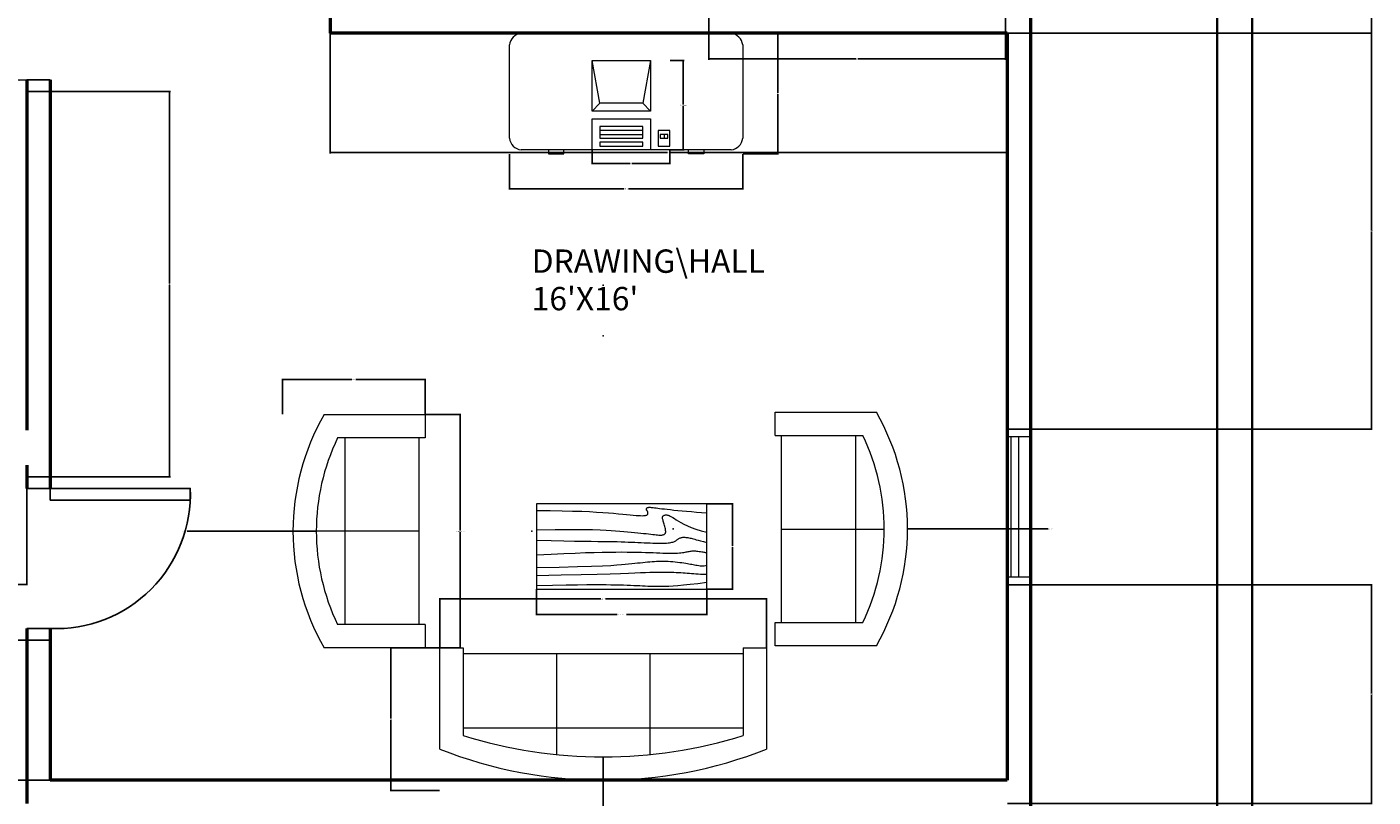
# Model space of a CAD drawing. Units: inches. Extents: x 156 to 720, y 11 to 679.
# Tile 3 of 5: x 374 to 720, y 161 to 359. Entities that reach past the tile are written whole.
import ezdxf

# ---------------------------------------------------------------- set-up
doc = ezdxf.new("R2010")
doc.units = ezdxf.units.IN
for name, color, linetype, lineweight in [('A-ANNO-DIMS', 2, 'Continuous', 18), ('A-AREA-IDEN', 7, 'Continuous', 25), ('A-DOOR', 3, 'Continuous', 25), ('A-EQPM', 9, 'Continuous', 13), ('A-FURN', 8, 'Continuous', 18), ('A-GLAZ', 4, 'Continuous', 18), ('A-WALL', 7, 'Continuous', 50), ('C-PROP', 7, 'Continuous', 35)]:
    doc.layers.add(name, color=color, linetype=linetype, lineweight=lineweight)
doc.styles.get("Standard").update_dxf_attribs({"font": 'arial.ttf'})
doc.dimstyles.get("Standard").update_dxf_attribs({"dimtxt": 0.18, "dimasz": 0.18, "dimexe": 0.18, "dimexo": 0.0625, "dimgap": 0.09, "dimtad": 0, "dimtih": 1, "dimtoh": 1, "dimdec": 4, "dimzin": 0, "dimdsep": 46, "dimtxsty": 'Standard', "dimcen": 0.09, "dimadec": 0, "dimazin": 0, "dimtfac": 1, "dimtdec": 4, "dimtofl": 0, "dimtmove": 0, "dimatfit": 3, "dimfxl": 1, "dimtolj": 1, "dimtzin": 0, "dimarcsym": 0})

# ---------------------------------------------------------------- blocks, each defined once
blk = doc.blocks.new('Sofa - Roundback Loveseat 5 ft.')
for p, q in [((0, -32.44198), (0, -5.99998)), ((-24, -33.99998), (-24, -11.46958)), ((-23.9998, -13.38178), (23.99986, -13.38178)), ((24.00004, -33.99998), (24.00004, -11.46958)), ((-24, -32.44198), (24.00004, -32.44198))]:
    blk.add_line(p, q)
for points in [[(-24, -33.99998), (-30, -33.99998), (-30, -7.99998)], [(30.00004, -7.99998), (30.00004, -33.99998), (24.00004, -33.99998)]]:
    blk.add_lwpolyline(points)
for centre, radius, start, end in [((0, -60.24998), 60.24998, 60.13715, 119.8628), ((0, -61.38438), 55.38444, 64.32083, 115.6792)]:
    blk.add_arc(centre, radius, start, end)
blk = doc.blocks.new('Table - Rectangular Woodgrain 60 x 30 in.')
for p, q in [((0, 0), (0, -30)), ((60, 0), (0, 0)), ((60, -30), (60, 0)), ((0, -30), (60, -30))]:
    blk.add_line(p, q)
for points in [[(0, -2.4), (4.8155, -2.418), (9.0302, -2.4688), (12.709, -2.5477), (15.9167, -2.65), (18.7181, -2.7711), (21.1781, -2.9063), (23.3616, -3.0508), (25.3333, -3.2), (27.1477, -3.3495), (28.8172, -3.4958), (30.3437, -3.636), (31.7291, -3.7667), (32.9756, -3.8849), (34.0849, -3.9875), (35.059, -4.0714), (35.9, -4.1334), (36.6114, -4.1711), (37.2041, -4.1854), (37.6906, -4.1779), (38.0833, -4.15), (38.3948, -4.1034), (38.6375, -4.0396), (38.8239, -3.9602), (38.9666, -3.8667), (39.0764, -3.7608), (39.1573, -3.6448), (39.2116, -3.521), (39.2416, -3.3917), (39.2498, -3.2593), (39.2385, -3.1261), (39.21, -2.9944), (39.1666, -2.8667), (39.111, -2.7447), (39.0468, -2.6281), (38.978, -2.5163), (38.9083, -2.4083), (38.8418, -2.3035), (38.7823, -2.201), (38.7337, -2.1001), (38.7, -2), (38.6844, -1.9003), (38.6875, -1.8021), (38.7094, -1.707), (38.75, -1.6167), (38.8094, -1.5326), (38.8875, -1.4563), (38.9844, -1.3893), (39.1, -1.3333), (39.2351, -1.2896), (39.3937, -1.2583), (39.5804, -1.2396), (39.8, -1.2333), (40.057, -1.2396), (40.3562, -1.2583), (40.7023, -1.2896), (41.1, -1.3333), (41.5547, -1.3895), (42.0755, -1.4573), (42.6721, -1.5361), (43.3542, -1.625), (44.1316, -1.7233), (45.014, -1.8302), (46.0114, -1.9449), (47.1333, -2.0667), (48.3862, -2.1947), (49.7625, -2.3281), (51.2513, -2.4663), (52.8416, -2.6083), (54.5226, -2.7535), (56.2833, -2.9011), (58.1127, -3.0501), (60, -3.2)], [(0, -9.2), (6.5759, -9.0858), (11.9385, -9.0365), (16.2527, -9.0418), (19.6833, -9.0917), (22.3952, -9.1759), (24.5531, -9.2844), (26.322, -9.4069), (27.8666, -9.5333), (29.3241, -9.6553), (30.7203, -9.7719), (32.0532, -9.8837), (33.3208, -9.9917), (34.5213, -10.0965), (35.6526, -10.199), (36.7128, -10.2999), (37.7, -10.4), (38.6129, -10.4996), (39.4531, -10.5969), (40.223, -10.6895), (40.925, -10.775), (41.5613, -10.8512), (42.1344, -10.9156), (42.6465, -10.966), (43.1, -11), (43.4976, -11.0158), (43.8437, -11.0136), (44.143, -10.9942), (44.4, -10.9583), (44.6195, -10.9069), (44.8062, -10.8406), (44.9648, -10.7603), (45.1, -10.6667), (45.2155, -10.5598), (45.3114, -10.4365), (45.3871, -10.2929), (45.4416, -10.125), (45.4743, -9.929), (45.4844, -9.7011), (45.4709, -9.4371), (45.4333, -9.1333), (45.3716, -8.7883), (45.2896, -8.4104), (45.1919, -8.0107), (45.0833, -7.6), (44.9685, -7.1893), (44.8521, -6.7896), (44.7388, -6.4117), (44.6333, -6.0667), (44.54, -5.7628), (44.4614, -5.4979), (44.4001, -5.2675), (44.3583, -5.0667), (44.3384, -4.8909), (44.3427, -4.7354), (44.3736, -4.5956), (44.4333, -4.4667), (44.5236, -4.3453), (44.6427, -4.2333), (44.7884, -4.1339), (44.9583, -4.05), (45.1501, -3.9849), (45.3614, -3.9417), (45.59, -3.9234), (45.8333, -3.9333), (46.0915, -3.9749), (46.3734, -4.0531), (46.6906, -4.1736), (47.0542, -4.3417), (47.4756, -4.5629), (47.9661, -4.8427), (48.5372, -5.1866), (49.2, -5.6), (49.9676, -6.0844), (50.8594, -6.625), (51.8965, -7.2031), (53.1, -7.8), (54.491, -8.3969), (56.0906, -8.975), (57.9199, -9.5156), (60, -10)], [(0, -12.8), (5.1847, -12.9322), (9.6213, -13.0323), (13.3963, -13.1059), (16.5958, -13.1583), (19.3063, -13.1952), (21.614, -13.2219), (23.6054, -13.2439), (25.3666, -13.2667), (26.9728, -13.2947), (28.4531, -13.3281), (29.8256, -13.3663), (31.1083, -13.4083), (32.3191, -13.4535), (33.476, -13.501), (34.597, -13.5501), (35.7, -13.6), (36.7984, -13.6497), (37.8875, -13.6979), (38.9578, -13.743), (40, -13.7833), (41.0047, -13.8174), (41.9625, -13.8438), (42.864, -13.8607), (43.7, -13.8667), (44.4631, -13.8604), (45.1552, -13.8417), (45.7801, -13.8104), (46.3416, -13.7667), (46.8439, -13.7104), (47.2906, -13.6417), (47.6858, -13.5604), (48.0333, -13.4667), (48.3375, -13.3608), (48.6042, -13.2448), (48.8396, -13.121), (49.05, -12.9917), (49.2417, -12.8593), (49.4208, -12.7261), (49.5937, -12.5944), (49.7667, -12.4667), (49.9452, -12.3451), (50.1323, -12.2313), (50.3303, -12.1268), (50.5416, -12.0333), (50.7686, -11.9524), (51.0135, -11.8854), (51.2788, -11.8341), (51.5666, -11.8), (51.8785, -11.7843), (52.2116, -11.7865), (52.562, -11.8059), (52.926, -11.8417), (53.2998, -11.8931), (53.6795, -11.9594), (54.0614, -12.0397), (54.4416, -12.1333), (54.8223, -12.2401), (55.2293, -12.3625), (55.6942, -12.5037), (56.2489, -12.6667), (56.9251, -12.8547), (57.7545, -13.0708), (58.7689, -13.3182), (60, -13.6)], [(0, -18), (5.124, -17.7273), (9.6609, -17.5057), (13.6705, -17.3303), (17.2125, -17.1958), (20.3467, -17.0973), (23.1328, -17.0297), (25.6307, -16.9878), (27.9, -16.9667), (29.9928, -16.9617), (31.9302, -16.9703), (33.7254, -16.9907), (35.3917, -17.0208), (36.9423, -17.0588), (38.3906, -17.1026), (39.7499, -17.1503), (41.0333, -17.2), (42.2519, -17.2496), (43.4073, -17.2969), (44.4986, -17.3395), (45.525, -17.375), (46.4858, -17.4012), (47.3802, -17.4156), (48.2074, -17.416), (48.9667, -17.4), (49.6583, -17.3662), (50.2872, -17.3167), (50.8595, -17.2547), (51.3812, -17.1833), (51.8584, -17.1057), (52.2971, -17.025), (52.7034, -16.9443), (53.0833, -16.8667), (53.443, -16.7951), (53.789, -16.7313), (54.128, -16.6768), (54.4666, -16.6334), (54.8115, -16.6024), (55.1693, -16.5854), (55.5465, -16.5841), (55.95, -16.6), (56.3828, -16.6337), (56.8346, -16.6823), (57.2915, -16.7418), (57.7396, -16.8084), (58.165, -16.878), (58.5539, -16.9469), (58.8924, -17.0111), (59.1666, -17.0667), (59.3679, -17.1107), (59.5078, -17.1438), (59.6032, -17.1675), (59.6708, -17.1833), (59.7275, -17.193), (59.7901, -17.1979), (59.8753, -17.1998), (60, -17.2)], [(0, -22.4), (8.0098, -22.2501), (14.4094, -22.1011), (19.4168, -21.9535), (23.25, -21.8083), (26.1269, -21.6663), (28.2656, -21.5281), (29.884, -21.3947), (31.2, -21.2667), (32.3967, -21.1448), (33.5172, -21.0292), (34.5697, -20.9198), (35.5625, -20.8167), (36.5037, -20.7198), (37.4015, -20.6292), (38.2642, -20.5448), (39.1, -20.4667), (39.9164, -20.3951), (40.7187, -20.3313), (41.5117, -20.2768), (42.3, -20.2333), (43.0883, -20.2024), (43.8812, -20.1854), (44.6836, -20.1841), (45.5, -20.2), (46.3328, -20.234), (47.1747, -20.2844), (48.0163, -20.3488), (48.8479, -20.425), (49.66, -20.5106), (50.4429, -20.6031), (51.1872, -20.7004), (51.8833, -20.8), (52.5246, -20.8999), (53.1166, -20.9995), (53.6681, -21.0983), (54.1875, -21.1958), (54.6834, -21.2919), (55.1646, -21.3859), (55.6394, -21.4777), (56.1167, -21.5667), (56.6028, -21.6515), (57.0961, -21.7266), (57.5929, -21.7852), (58.0896, -21.8208), (58.5823, -21.8268), (59.0674, -21.7964), (59.5412, -21.723), (60, -21.6)], [(0, -25.2), (8.6355, -25.0504), (15.7026, -24.9031), (21.4049, -24.7606), (25.9458, -24.625), (29.529, -24.4988), (32.3578, -24.3844), (34.6359, -24.284), (36.5667, -24.2), (38.3213, -24.1341), (39.9417, -24.0854), (41.437, -24.0523), (42.8167, -24.0333), (44.0901, -24.0268), (45.2667, -24.0313), (46.3557, -24.0451), (47.3667, -24.0667), (48.309, -24.0947), (49.1928, -24.1287), (50.0284, -24.168), (50.826, -24.2125), (51.5959, -24.2617), (52.3483, -24.3151), (53.0935, -24.3725), (53.8417, -24.4334), (54.6009, -24.497), (55.3699, -24.561), (56.1454, -24.6226), (56.9239, -24.6792), (57.7021, -24.7279), (58.4764, -24.7662), (59.2435, -24.7911), (60, -24.8)], [(0, -28.8), (5.6867, -28.6681), (10.45, -28.5698), (14.407, -28.5012), (17.675, -28.4584), (20.3711, -28.4374), (22.6125, -28.4344), (24.5164, -28.4455), (26.2, -28.4667), (27.762, -28.4947), (29.2276, -28.5281), (30.6033, -28.5663), (31.8958, -28.6084), (33.1118, -28.6535), (34.2578, -28.7011), (35.3405, -28.7501), (36.3666, -28.8), (37.3443, -28.8497), (38.288, -28.8974), (39.2137, -28.9412), (40.1375, -28.9792), (41.0753, -29.0093), (42.0432, -29.0297), (43.0572, -29.0384), (44.1333, -29.0333), (45.2936, -29.0114), (46.5843, -28.9641), (48.0579, -28.8816), (49.7666, -28.7542), (51.7629, -28.5721), (54.0989, -28.3255), (56.8272, -28.0048), (60, -27.6)]]:
    blk.add_lwpolyline(points)
blk = doc.blocks.new('Sofa - Roundback 7 ft.')
for p, q in [((-12.00002, -32.4421), (-12.00003, -6.5971)), ((11.99997, -32.4421), (11.99998, -6.5971)), ((-36.000027, -34), (-36.000027, -11.4696)), ((-35.999844, -13.3819), (35.9998, -13.3819)), ((35.99998, -34), (35.99998, -11.4696)), ((-36.000027, -32.4421), (35.99998, -32.4421))]:
    blk.add_line(p, q)
for points in [[(-36.000027, -34), (-42.000027, -34), (-42.000027, -8)], [(41.99998, -8), (41.99998, -34), (35.99998, -34)]]:
    blk.add_lwpolyline(points)
for centre, radius, start, end in [((0, -114.25), 114.25, 68.43141, 111.5686), ((-0.00001, -127.1968), 121.1968, 72.72033, 107.2797)]:
    blk.add_arc(centre, radius, start, end)
blk = doc.blocks.new('Desk - 30 x 60 in.')
for p, q in [((-26.999995, 0), (26.999995, 0)), ((-29.999995, -27), (-29.999995, -3)), ((29.999995, -3), (29.999995, -27)), ((26.999995, -30), (-26.999995, -30)), ((-20.000005, -30), (-20.000005, -31)), ((-20.000005, -31), (-16.000005, -31)), ((-16.000005, -31), (-16.000005, -30)), ((15.999995, -31), (15.999995, -30)), ((19.999995, -31), (15.999995, -31)), ((19.999995, -30), (19.999995, -31))]:
    blk.add_line(p, q)
for centre, start, end in [((-26.499995, -3.5), 98.1301, 171.8699), ((26.499995, -3.5), 8.130102, 81.8699), ((-26.499995, -26.5), 188.1301, 261.8699), ((26.499995, -26.5), 278.1301, 351.8699)]:
    blk.add_arc(centre, 3.535534, start, end)
blk = doc.blocks.new('Computer Terminal')
for p, q in [((-10, 11.5), (5, 11.5)), ((-8, 0.5), (-10, 11.5)), ((-10, -1.5), (-10, 11.5)), ((5, 11.5), (3, 0.5)), ((5, 11.5), (5, -1.5)), ((-10, -1.5), (-8, 0.5)), ((3, 0.5), (-8, 0.5)), ((3, 0.5), (5, -1.5)), ((5, -1.5), (-10, -1.5)), ((-10, -11.5), (-10, -3.5)), ((-10, -3.5), (5, -3.5)), ((-8, -5.5), (-8, -8.5)), ((3, -5.5), (-8, -5.5)), ((3, -6.5), (-8, -6.5)), ((3, -8.5), (3, -5.5)), ((5, -3.5), (5, -11.5)), ((10, -6.5), (7, -6.5)), ((7, -6.5), (7, -10.5)), ((10, -10.5), (10, -6.5)), ((-8, -7.5), (3, -7.5)), ((-8, -8.5), (3, -8.5)), ((-8, -9.5), (-8, -10.5)), ((3, -9.5), (-8, -9.5)), ((3, -10.5), (3, -9.5)), ((9.5, -7.5), (7.5, -7.5)), ((7.5, -7.5), (7.5, -8.5)), ((7.5, -8.5), (9.5, -8.5)), ((8.5, -7.5), (8.5, -8.5)), ((9.5, -8.5), (9.5, -7.5)), ((5, -11.5), (-10, -11.5)), ((-8, -10.5), (3, -10.5)), ((7, -10.5), (10, -10.5))]:
    blk.add_line(p, q)
blk = doc.blocks.new('DOOR-SWING-36IN')
for p, q in [((0, 6), (0, 0)), ((3, 6), (3, 0)), ((39, 6), (39, 0)), ((42, 6), (42, 0))]:
    blk.add_line(p, q)
blk.add_lwpolyline([(39, 6), (36, 6), (36, 42), (39, 42)], close=True)
blk.add_arc((37.5, 7.5), 34.53, 87.5104, 182.4896)
blk = doc.blocks.new('WIN-36IN-WALL6')
for p, q in [((6, 40), (0, 40)), ((6, 38), (0, 38)), ((0, 38), (0, 2)), ((1, 2), (1, 38)), ((3, 2), (3, 38)), ((6, 2), (6, 38)), ((0, 2), (6, 2)), ((0, 0), (6, 0))]:
    blk.add_line(p, q)
blk = doc.blocks.new('*D35')
at = {"layer": 'A-ANNO-DIMS', "color": 0, "lineweight": -2, "transparency": 16777216}
for p, q in [((476.19, 259.15), (485.31, 259.15)), ((485.13, 258.97), (485.13, 229.33)), ((485.13, 199.33), (485.13, 228.97)), ((476.19, 199.15), (485.31, 199.15))]:
    blk.add_line(p, q, dxfattribs=at)
at = {"layer": 'A-ANNO-DIMS', "color": 0, "transparency": 16777216}
for points in [[(485.1, 258.97), (485.16, 258.97), (485.13, 259.15)], [(485.1, 199.33), (485.16, 199.33), (485.13, 199.15)]]:
    blk.add_solid(points, dxfattribs=at)
at = {"layer": 'Defpoints', "color": 0, "transparency": 16777216}
for p in [(476.13, 259.15), (485.13, 259.15), (476.13, 199.15)]:
    blk.add_point(p, dxfattribs=at)
at = {"layer": 'A-ANNO-DIMS', "color": 0, "transparency": 16777216, "insert": (485.13, 229.15), "char_height": 0.18, "attachment_point": 5}
blk.add_mtext('\\A1;LOVESEAT 60 TYP.', dxfattribs=at)
blk = doc.blocks.new('*D36')
at = {"layer": 'A-ANNO-DIMS', "color": 0, "lineweight": -2, "transparency": 16777216}
for p, q in [((439.46, 259.21), (439.46, 268.33)), ((439.64, 268.15), (457.26, 268.15)), ((475.95, 268.15), (458.32, 268.15)), ((476.13, 259.21), (476.13, 268.33))]:
    blk.add_line(p, q, dxfattribs=at)
at = {"layer": 'A-ANNO-DIMS', "color": 0, "transparency": 16777216}
for points in [[(439.64, 268.18), (439.64, 268.12), (439.46, 268.15)], [(475.95, 268.18), (475.95, 268.12), (476.13, 268.15)]]:
    blk.add_solid(points, dxfattribs=at)
at = {"layer": 'Defpoints', "color": 0, "transparency": 16777216}
for p in [(439.46, 268.15), (439.46, 259.15), (476.13, 259.15)]:
    blk.add_point(p, dxfattribs=at)
at = {"layer": 'A-ANNO-DIMS', "color": 0, "transparency": 16777216, "insert": (457.79, 268.15), "char_height": 0.18, "attachment_point": 5}
blk.add_mtext('\\A1;37 TYP.', dxfattribs=at)
blk = doc.blocks.new('*D38')
at = {"layer": 'A-ANNO-DIMS', "color": 0, "lineweight": -2, "transparency": 16777216}
for p, q in [((549.06, 363.36), (549.06, 350.35)), ((625.27, 363.36), (625.27, 350.35)), ((549.24, 350.53), (586.94, 350.53)), ((625.09, 350.53), (587.38, 350.53))]:
    blk.add_line(p, q, dxfattribs=at)
at = {"layer": 'A-ANNO-DIMS', "color": 0, "transparency": 16777216}
for points in [[(549.24, 350.56), (549.24, 350.5), (549.06, 350.53)], [(625.09, 350.56), (625.09, 350.5), (625.27, 350.53)]]:
    blk.add_solid(points, dxfattribs=at)
at = {"layer": 'Defpoints', "color": 0, "transparency": 16777216}
for p in [(549.06, 363.42), (625.27, 363.42), (625.27, 350.53)]:
    blk.add_point(p, dxfattribs=at)
at = {"layer": 'A-ANNO-DIMS', "color": 0, "transparency": 16777216, "insert": (587.16, 350.53), "char_height": 0.18, "attachment_point": 5}
blk.add_mtext('\\A1;76', dxfattribs=at)
blk = doc.blocks.new('*D39')
at = {"layer": 'A-ANNO-DIMS', "color": 0, "lineweight": -2, "transparency": 16777216}
for p, q in [((504.72, 214.23), (504.72, 207.53)), ((548.55, 214.23), (548.55, 207.53)), ((504.9, 207.71), (525.44, 207.71)), ((548.37, 207.71), (527.83, 207.71))]:
    blk.add_line(p, q, dxfattribs=at)
at = {"layer": 'A-ANNO-DIMS', "color": 0, "transparency": 16777216}
for points in [[(504.9, 207.74), (504.9, 207.68), (504.72, 207.71)], [(548.37, 207.74), (548.37, 207.68), (548.55, 207.71)]]:
    blk.add_solid(points, dxfattribs=at)
at = {"layer": 'Defpoints', "color": 0, "transparency": 16777216}
for p in [(504.72, 214.29), (548.55, 214.29), (548.55, 207.71)]:
    blk.add_point(p, dxfattribs=at)
at = {"layer": 'A-ANNO-DIMS', "color": 0, "transparency": 16777216, "insert": (526.63, 207.71), "char_height": 0.18, "attachment_point": 5}
blk.add_mtext('\\A1;COFFEE TABLE 44', dxfattribs=at)
blk = doc.blocks.new('*D40')
at = {"layer": 'A-ANNO-DIMS', "color": 0, "lineweight": -2, "transparency": 16777216}
for p, q in [((548.61, 236.2), (555.3, 236.2)), ((555.12, 236.02), (555.12, 225.42)), ((555.12, 214.47), (555.12, 225.06)), ((548.61, 214.29), (555.3, 214.29))]:
    blk.add_line(p, q, dxfattribs=at)
at = {"layer": 'A-ANNO-DIMS', "color": 0, "transparency": 16777216}
for points in [[(555.09, 236.02), (555.15, 236.02), (555.12, 236.2)], [(555.09, 214.47), (555.15, 214.47), (555.12, 214.29)]]:
    blk.add_solid(points, dxfattribs=at)
at = {"layer": 'Defpoints', "color": 0, "transparency": 16777216}
for p in [(548.55, 236.2), (555.12, 236.2), (548.55, 214.29)]:
    blk.add_point(p, dxfattribs=at)
at = {"layer": 'A-ANNO-DIMS', "color": 0, "transparency": 16777216, "insert": (555.12, 225.24), "char_height": 0.18, "attachment_point": 5}
blk.add_mtext('\\A1;22', dxfattribs=at)
blk = doc.blocks.new('*D43')
at = {"layer": 'A-ANNO-DIMS', "color": 0, "lineweight": -2, "transparency": 16777216}
for p, q in [((479.88, 199.21), (479.88, 211.93)), ((480.06, 211.75), (521.29, 211.75)), ((563.7, 211.75), (522.48, 211.75)), ((563.88, 199.21), (563.88, 211.93))]:
    blk.add_line(p, q, dxfattribs=at)
at = {"layer": 'A-ANNO-DIMS', "color": 0, "transparency": 16777216}
for points in [[(480.06, 211.78), (480.06, 211.72), (479.88, 211.75)], [(563.7, 211.78), (563.7, 211.72), (563.88, 211.75)]]:
    blk.add_solid(points, dxfattribs=at)
at = {"layer": 'Defpoints', "color": 0, "transparency": 16777216}
for p in [(479.88, 211.75), (479.88, 199.15), (563.88, 199.15)]:
    blk.add_point(p, dxfattribs=at)
at = {"layer": 'A-ANNO-DIMS', "color": 0, "transparency": 16777216, "insert": (521.88, 211.75), "char_height": 0.18, "attachment_point": 5}
blk.add_mtext('\\A1;SOFA 84', dxfattribs=at)
blk = doc.blocks.new('*D44')
at = {"layer": 'A-ANNO-DIMS', "color": 0, "lineweight": -2, "transparency": 16777216}
for p, q in [((479.82, 199.15), (467.1, 199.15)), ((467.28, 198.97), (467.28, 181)), ((467.28, 162.66), (467.28, 180.64)), ((479.82, 162.48), (467.1, 162.48))]:
    blk.add_line(p, q, dxfattribs=at)
at = {"layer": 'A-ANNO-DIMS', "color": 0, "transparency": 16777216}
for points in [[(467.25, 198.97), (467.31, 198.97), (467.28, 199.15)], [(467.25, 162.66), (467.31, 162.66), (467.28, 162.48)]]:
    blk.add_solid(points, dxfattribs=at)
at = {"layer": 'Defpoints', "color": 0, "transparency": 16777216}
for p in [(479.88, 199.15), (467.28, 162.48), (479.88, 162.48)]:
    blk.add_point(p, dxfattribs=at)
at = {"layer": 'A-ANNO-DIMS', "color": 0, "transparency": 16777216, "insert": (467.28, 180.82), "char_height": 0.18, "attachment_point": 5}
blk.add_mtext('\\A1;37', dxfattribs=at)
blk = doc.blocks.new('*D45')
at = {"layer": 'A-ANNO-DIMS', "color": 0, "lineweight": -2, "transparency": 16777216}
for p, q in [((497.77, 326.09), (497.77, 316.97)), ((557.77, 326.09), (557.77, 316.97)), ((497.95, 317.15), (527.18, 317.15)), ((557.59, 317.15), (528.36, 317.15))]:
    blk.add_line(p, q, dxfattribs=at)
at = {"layer": 'A-ANNO-DIMS', "color": 0, "transparency": 16777216}
for points in [[(497.95, 317.18), (497.95, 317.12), (497.77, 317.15)], [(557.59, 317.18), (557.59, 317.12), (557.77, 317.15)]]:
    blk.add_solid(points, dxfattribs=at)
at = {"layer": 'Defpoints', "color": 0, "transparency": 16777216}
for p in [(497.77, 326.15), (557.77, 326.15), (557.77, 317.15)]:
    blk.add_point(p, dxfattribs=at)
at = {"layer": 'A-ANNO-DIMS', "color": 0, "transparency": 16777216, "insert": (527.77, 317.15), "char_height": 0.18, "attachment_point": 5}
blk.add_mtext('\\A1;DESK 60', dxfattribs=at)
blk = doc.blocks.new('*D46')
at = {"layer": 'A-ANNO-DIMS', "color": 0, "lineweight": -2, "transparency": 16777216}
for p, q in [((557.83, 357.15), (566.95, 357.15)), ((566.77, 356.97), (566.77, 341.83)), ((566.77, 326.33), (566.77, 341.47)), ((557.83, 326.15), (566.95, 326.15))]:
    blk.add_line(p, q, dxfattribs=at)
at = {"layer": 'A-ANNO-DIMS', "color": 0, "transparency": 16777216}
for points in [[(566.74, 356.97), (566.8, 356.97), (566.77, 357.15)], [(566.74, 326.33), (566.8, 326.33), (566.77, 326.15)]]:
    blk.add_solid(points, dxfattribs=at)
at = {"layer": 'Defpoints', "color": 0, "transparency": 16777216}
for p in [(557.77, 357.15), (566.77, 357.15), (557.77, 326.15)]:
    blk.add_point(p, dxfattribs=at)
at = {"layer": 'A-ANNO-DIMS', "color": 0, "transparency": 16777216, "insert": (566.77, 341.65), "char_height": 0.18, "attachment_point": 5}
blk.add_mtext('\\A1;31', dxfattribs=at)
blk = doc.blocks.new('*D47')
at = {"layer": 'A-ANNO-DIMS', "color": 0, "lineweight": -2, "transparency": 16777216}
for p, q in [((539.09, 350.15), (542.65, 350.15)), ((542.47, 349.97), (542.47, 338.83)), ((542.47, 327.33), (542.47, 338.47)), ((539.09, 327.15), (542.65, 327.15))]:
    blk.add_line(p, q, dxfattribs=at)
at = {"layer": 'A-ANNO-DIMS', "color": 0, "transparency": 16777216}
for points in [[(542.44, 349.97), (542.5, 349.97), (542.47, 350.15)], [(542.44, 327.33), (542.5, 327.33), (542.47, 327.15)]]:
    blk.add_solid(points, dxfattribs=at)
at = {"layer": 'Defpoints', "color": 0, "transparency": 16777216}
for p in [(539.02, 350.15), (542.47, 350.15), (539.02, 327.15)]:
    blk.add_point(p, dxfattribs=at)
at = {"layer": 'A-ANNO-DIMS', "color": 0, "transparency": 16777216, "insert": (542.47, 338.65), "char_height": 0.18, "attachment_point": 5}
blk.add_mtext('\\A1;COMPUTER 23', dxfattribs=at)
blk = doc.blocks.new('*D48')
at = {"layer": 'A-ANNO-DIMS', "color": 0, "lineweight": -2, "transparency": 16777216}
for p, q in [((519.02, 327.09), (519.02, 323.52)), ((539.02, 327.09), (539.02, 323.52)), ((519.2, 323.7), (528.8, 323.7)), ((538.84, 323.7), (529.24, 323.7))]:
    blk.add_line(p, q, dxfattribs=at)
at = {"layer": 'A-ANNO-DIMS', "color": 0, "transparency": 16777216}
for points in [[(519.2, 323.73), (519.2, 323.67), (519.02, 323.7)], [(538.84, 323.73), (538.84, 323.67), (539.02, 323.7)]]:
    blk.add_solid(points, dxfattribs=at)
at = {"layer": 'Defpoints', "color": 0, "transparency": 16777216}
for p in [(519.02, 327.15), (539.02, 327.15), (539.02, 323.7)]:
    blk.add_point(p, dxfattribs=at)
at = {"layer": 'A-ANNO-DIMS', "color": 0, "transparency": 16777216, "insert": (529.02, 323.7), "char_height": 0.18, "attachment_point": 5}
blk.add_mtext('\\A1;20', dxfattribs=at)
blk = doc.blocks.new('*D60')
at = {"layer": 'A-ANNO-DIMS', "color": 0, "lineweight": -2, "transparency": 16777216}
for p, q in [((625.79, 215.4), (719.6, 215.4)), ((719.42, 215.22), (719.42, 187.46)), ((719.42, 159.33), (719.42, 187.09)), ((625.79, 159.15), (719.6, 159.15))]:
    blk.add_line(p, q, dxfattribs=at)
at = {"layer": 'A-ANNO-DIMS', "color": 0, "transparency": 16777216}
for points in [[(719.39, 215.22), (719.45, 215.22), (719.42, 215.4)], [(719.39, 159.33), (719.45, 159.33), (719.42, 159.15)]]:
    blk.add_solid(points, dxfattribs=at)
at = {"layer": 'Defpoints', "color": 0, "transparency": 16777216}
for p in [(625.72, 215.4), (719.42, 215.4), (625.72, 159.15)]:
    blk.add_point(p, dxfattribs=at)
at = {"layer": 'A-ANNO-DIMS', "color": 0, "transparency": 16777216, "insert": (719.42, 187.27), "char_height": 0.18, "attachment_point": 5}
blk.add_mtext('\\A1;56.25', dxfattribs=at)
blk = doc.blocks.new('*D61')
at = {"layer": 'A-ANNO-DIMS', "color": 0, "lineweight": -2, "transparency": 16777216}
for p, q in [((625.79, 357.15), (719.6, 357.15)), ((719.42, 356.97), (719.42, 306.46)), ((719.42, 255.58), (719.42, 306.09)), ((625.79, 255.4), (719.6, 255.4))]:
    blk.add_line(p, q, dxfattribs=at)
at = {"layer": 'A-ANNO-DIMS', "color": 0, "transparency": 16777216}
for points in [[(719.39, 356.97), (719.45, 356.97), (719.42, 357.15)], [(719.39, 255.58), (719.45, 255.58), (719.42, 255.4)]]:
    blk.add_solid(points, dxfattribs=at)
at = {"layer": 'Defpoints', "color": 0, "transparency": 16777216}
for p in [(625.72, 357.15), (719.42, 357.15), (625.72, 255.4)]:
    blk.add_point(p, dxfattribs=at)
at = {"layer": 'A-ANNO-DIMS', "color": 0, "transparency": 16777216, "insert": (719.42, 306.27), "char_height": 0.18, "attachment_point": 5}
blk.add_mtext('\\A1;101.75', dxfattribs=at)
blk = doc.blocks.new('*D62')
at = {"layer": 'A-ANNO-DIMS', "color": 0, "lineweight": -2, "transparency": 16777216}
for p, q in [((625.79, 450.15), (719.6, 450.15)), ((719.42, 449.97), (719.42, 403.83)), ((719.42, 357.33), (719.42, 403.47)), ((625.79, 357.15), (719.6, 357.15))]:
    blk.add_line(p, q, dxfattribs=at)
at = {"layer": 'A-ANNO-DIMS', "color": 0, "transparency": 16777216}
for points in [[(719.39, 449.97), (719.45, 449.97), (719.42, 450.15)], [(719.39, 357.33), (719.45, 357.33), (719.42, 357.15)]]:
    blk.add_solid(points, dxfattribs=at)
at = {"layer": 'Defpoints', "color": 0, "transparency": 16777216}
for p in [(625.72, 450.15), (719.42, 450.15), (625.72, 357.15)]:
    blk.add_point(p, dxfattribs=at)
at = {"layer": 'A-ANNO-DIMS', "color": 0, "transparency": 16777216, "insert": (719.42, 403.65), "char_height": 0.18, "attachment_point": 5}
blk.add_mtext('\\A1;93', dxfattribs=at)
blk = doc.blocks.new('*D68')
at = {"layer": 'A-ANNO-DIMS', "color": 0, "lineweight": -2, "transparency": 16777216}
for p, q in [((379.66, 201.15), (348.84, 201.15)), ((349.02, 200.97), (349.02, 183.33)), ((349.02, 165.33), (349.02, 182.97)), ((379.66, 165.15), (348.84, 165.15))]:
    blk.add_line(p, q, dxfattribs=at)
at = {"layer": 'A-ANNO-DIMS', "color": 0, "transparency": 16777216}
for points in [[(348.99, 200.97), (349.05, 200.97), (349.02, 201.15)], [(348.99, 165.33), (349.05, 165.33), (349.02, 165.15)]]:
    blk.add_solid(points, dxfattribs=at)
at = {"layer": 'Defpoints', "color": 0, "transparency": 16777216}
for p in [(349.02, 201.15), (379.72, 201.15), (379.72, 165.15)]:
    blk.add_point(p, dxfattribs=at)
at = {"layer": 'A-ANNO-DIMS', "color": 0, "transparency": 16777216, "insert": (349.02, 183.15), "char_height": 0.18, "attachment_point": 5}
blk.add_mtext('\\A1;36', dxfattribs=at)
blk = doc.blocks.new('*D69')
at = {"layer": 'A-ANNO-DIMS', "color": 0, "lineweight": -2, "transparency": 16777216}
for p, q in [((379.79, 342.15), (410.6, 342.15)), ((410.42, 341.97), (410.42, 292.83)), ((410.42, 243.33), (410.42, 292.47)), ((379.79, 243.15), (410.6, 243.15))]:
    blk.add_line(p, q, dxfattribs=at)
at = {"layer": 'A-ANNO-DIMS', "color": 0, "transparency": 16777216}
for points in [[(410.39, 341.97), (410.45, 341.97), (410.42, 342.15)], [(410.39, 243.33), (410.45, 243.33), (410.42, 243.15)]]:
    blk.add_solid(points, dxfattribs=at)
at = {"layer": 'Defpoints', "color": 0, "transparency": 16777216}
for p in [(379.72, 342.15), (379.72, 243.15), (410.42, 243.15)]:
    blk.add_point(p, dxfattribs=at)
at = {"layer": 'A-ANNO-DIMS', "color": 0, "transparency": 16777216, "insert": (410.42, 292.65), "char_height": 0.18, "attachment_point": 5}
blk.add_mtext('\\A1;99', dxfattribs=at)
blk = doc.blocks.new('*D74')
at = {"layer": 'A-ANNO-DIMS', "color": 0, "lineweight": -2, "transparency": 16777216}
for p, q in [((326.1, 246.09), (326.1, 215.27)), ((373.72, 246.09), (373.72, 215.27)), ((326.28, 215.45), (349.52, 215.45)), ((373.54, 215.45), (350.31, 215.45))]:
    blk.add_line(p, q, dxfattribs=at)
at = {"layer": 'A-ANNO-DIMS', "color": 0, "transparency": 16777216}
for points in [[(326.28, 215.48), (326.28, 215.42), (326.1, 215.45)], [(373.54, 215.48), (373.54, 215.42), (373.72, 215.45)]]:
    blk.add_solid(points, dxfattribs=at)
at = {"layer": 'Defpoints', "color": 0, "transparency": 16777216}
for p in [(326.1, 246.15), (373.72, 246.15), (326.1, 215.45)]:
    blk.add_point(p, dxfattribs=at)
at = {"layer": 'A-ANNO-DIMS', "color": 0, "transparency": 16777216, "insert": (349.91, 215.45), "char_height": 0.18, "attachment_point": 5}
blk.add_mtext('\\A1;47.62', dxfattribs=at)
blk = doc.blocks.new('*D79')
at = {"layer": 'A-ANNO-DIMS', "color": 0, "lineweight": -2, "transparency": 16777216}
for p, q in [((451.72, 357.09), (451.72, 326.27)), ((625.72, 357.09), (625.72, 326.27)), ((451.9, 326.45), (538.44, 326.45)), ((625.54, 326.45), (539, 326.45))]:
    blk.add_line(p, q, dxfattribs=at)
at = {"layer": 'A-ANNO-DIMS', "color": 0, "transparency": 16777216}
for points in [[(451.9, 326.48), (451.9, 326.42), (451.72, 326.45)], [(625.54, 326.48), (625.54, 326.42), (625.72, 326.45)]]:
    blk.add_solid(points, dxfattribs=at)
at = {"layer": 'Defpoints', "color": 0, "transparency": 16777216}
for p in [(451.72, 357.15), (625.72, 357.15), (451.72, 326.45)]:
    blk.add_point(p, dxfattribs=at)
at = {"layer": 'A-ANNO-DIMS', "color": 0, "transparency": 16777216, "insert": (538.72, 326.45), "char_height": 0.18, "attachment_point": 5}
blk.add_mtext('\\A1;174', dxfattribs=at)
blk = doc.blocks.new('*D81')
at = {"layer": 'A-ANNO-DIMS', "color": 0, "lineweight": -2, "transparency": 16777216}
for p, q in [((521.79, 292.35), (521.97, 292.35)), ((521.88, 292.26), (521.88, 292.44)), ((521.88, 98.43), (521.88, 170.97)), ((521.7, 98.43), (521.88, 98.43))]:
    blk.add_line(p, q, dxfattribs=at)
at = {"layer": 'A-ANNO-DIMS', "color": 0, "transparency": 16777216}
blk.add_solid([(521.85, 170.97), (521.91, 170.97), (521.88, 171.15)], dxfattribs=at)
at = {"layer": 'Defpoints', "color": 0, "transparency": 16777216}
for p in [(521.88, 292.35), (521.88, 171.15)]:
    blk.add_point(p, dxfattribs=at)
at = {"layer": 'A-ANNO-DIMS', "color": 0, "transparency": 16777216, "insert": (521.22, 98.43), "char_height": 0.18, "attachment_point": 5}
blk.add_mtext('\\A1;R121.2', dxfattribs=at)
blk = doc.blocks.new('*D82')
at = {"layer": 'A-ANNO-DIMS', "color": 0, "lineweight": -2, "transparency": 16777216}
for p, q in [((521.79, 279.4), (521.97, 279.4)), ((521.88, 279.31), (521.88, 279.49)), ((521.88, 96.6), (521.88, 164.97)), ((521.7, 96.6), (521.88, 96.6))]:
    blk.add_line(p, q, dxfattribs=at)
at = {"layer": 'A-ANNO-DIMS', "color": 0, "transparency": 16777216}
blk.add_solid([(521.85, 164.97), (521.91, 164.97), (521.88, 165.15)], dxfattribs=at)
at = {"layer": 'Defpoints', "color": 0, "transparency": 16777216}
for p in [(521.88, 279.4), (521.88, 165.15)]:
    blk.add_point(p, dxfattribs=at)
at = {"layer": 'A-ANNO-DIMS', "color": 0, "transparency": 16777216, "insert": (521.15, 96.6), "char_height": 0.18, "attachment_point": 5}
blk.add_mtext('\\A1;R114.25', dxfattribs=at)
blk = doc.blocks.new('*D83')
at = {"layer": 'A-ANNO-DIMS', "color": 0, "lineweight": -2, "transparency": 16777216}
for p, q in [((539.76, 229.72), (539.94, 229.72)), ((539.85, 229.63), (539.85, 229.81)), ((636.25, 229.72), (600.28, 229.72))]:
    blk.add_line(p, q, dxfattribs=at)
at = {"layer": 'A-ANNO-DIMS', "color": 0, "transparency": 16777216}
blk.add_solid([(600.28, 229.75), (600.28, 229.69), (600.1, 229.72)], dxfattribs=at)
at = {"layer": 'Defpoints', "color": 0, "transparency": 16777216}
for p in [(539.85, 229.72), (600.1, 229.72)]:
    blk.add_point(p, dxfattribs=at)
at = {"layer": 'A-ANNO-DIMS', "color": 0, "transparency": 16777216, "insert": (636.93, 229.72), "char_height": 0.18, "attachment_point": 5}
blk.add_mtext('\\A1;2X R60.25', dxfattribs=at)
blk = doc.blocks.new('*D84')
at = {"layer": 'A-ANNO-DIMS', "color": 0, "lineweight": -2, "transparency": 16777216}
for p, q in [((414.9, 229.15), (447.95, 229.15)), ((503.42, 229.15), (503.6, 229.15)), ((503.51, 229.06), (503.51, 229.24))]:
    blk.add_line(p, q, dxfattribs=at)
at = {"layer": 'A-ANNO-DIMS', "color": 0, "transparency": 16777216}
blk.add_solid([(447.95, 229.18), (447.95, 229.12), (448.13, 229.15)], dxfattribs=at)
at = {"layer": 'Defpoints', "color": 0, "transparency": 16777216}
for p in [(448.13, 229.15), (503.51, 229.15)]:
    blk.add_point(p, dxfattribs=at)
at = {"layer": 'A-ANNO-DIMS', "color": 0, "transparency": 16777216, "insert": (414.22, 229.15), "char_height": 0.18, "attachment_point": 5}
blk.add_mtext('\\A1;2X R55.38', dxfattribs=at)

msp = doc.modelspace()

# ---------------------------------------------------------------- linework, layer by layer
at = {"layer": 'A-WALL'}
for p, q in [((631.7236, 453.1514), (631.7236, 80.1514)), ((451.7236, 363.1514), (451.7236, 357.1514)), ((625.7236, 357.1514), (451.7236, 357.1514)), ((625.7236, 357.1514), (625.7236, 165.1514)), ((373.7236, 345.1514), (373.7236, 255.1514)), ((379.7236, 345.1514), (379.7236, 246.1514)), ((373.7236, 246.1514), (373.7236, 240.1514)), ((379.7236, 246.1514), (379.7236, 240.1514)), ((373.7236, 204.1514), (373.7236, 159.1514)), ((379.7236, 204.1514), (379.7236, 165.1514)), ((625.7236, 165.1514), (379.7236, 165.1514))]:
    msp.add_line(p, q, dxfattribs=at)
at = {"layer": 'C-PROP'}
for p, q in [((688.7236, 42.1514), (688.7236, 642.1514)), ((679.7236, 51.1514), (679.7236, 543.1514))]:
    msp.add_line(p, q, dxfattribs=at)

# ---------------------------------------------------------------- block references
at = {"layer": 'A-DOOR', "rotation": 89.99999999999989}
msp.add_blockref('DOOR-SWING-36IN', (379.724, 342.1518), dxfattribs=at)
at = {"layer": 'A-DOOR', "extrusion": (0, 0, -1), "zscale": -1, "rotation": 89.99999999999999}
msp.add_blockref('DOOR-SWING-36IN', (-373.7232, 201.1518), dxfattribs=at)
at = {"layer": 'A-EQPM'}
msp.add_blockref('Computer Terminal', (529.0227, 338.6514), dxfattribs=at)
at = {"layer": 'A-FURN'}
msp.add_blockref('Desk - 30 x 60 in.', (527.7713, 357.1514), dxfattribs=at)
for name, p, rotation in [('Sofa - Roundback Loveseat 5 ft.', (600.1048, 229.7163), 270), ('Sofa - Roundback Loveseat 5 ft.', (442.1263, 229.1514), 90), ('Sofa - Roundback 7 ft.', (521.881, 165.1514), 180)]:
    msp.add_blockref(name, p, dxfattribs=dict(at, rotation=rotation))
at = {"layer": 'A-FURN', "xscale": 0.7303618039707552, "yscale": 0.7303618039707552, "zscale": 0.7303618039707552}
msp.add_blockref('Table - Rectangular Woodgrain 60 x 30 in.', (504.7235, 236.199), dxfattribs=at)
at = {"layer": 'A-GLAZ'}
msp.add_blockref('WIN-36IN-WALL6', (625.724, 215.3973), dxfattribs=at)

# ---------------------------------------------------------------- texts
at = {"layer": 'A-AREA-IDEN'}
for s, p in [('DRAWING\\HALL', (503.4842, 295.5662)), ("16'X16'", (503.4842, 285.9277))]:
    msp.add_text(s, height=6, dxfattribs=at).set_placement(p)

# ---------------------------------------------------------------- dimensions: what is measured, and where the dimension line sits
at = {"layer": 'A-ANNO-DIMS'}
for base, p1, p2, angle, override, picture, middle in [((719.4236, 450.1514), (625.7236, 357.1514), (625.7236, 450.1514), 90, {"dimdec": 0, "dimlfac": 1, "dimrnd": 0, "dimzin": 0, "dimdsep": 46, "dimlunit": 2}, '*D62', (719.4236, 403.6514)), ((451.7236, 326.4514), (625.7236, 357.1514), (451.7236, 357.1514), 180, {"dimdec": 0, "dimlfac": 1, "dimrnd": 0, "dimzin": 0, "dimdsep": 46, "dimlunit": 2}, '*D79', (538.7236, 326.4514)), ((566.7713, 357.1514), (557.7713, 326.1514), (557.7713, 357.1514), 90, {"dimdec": 0, "dimlfac": 1, "dimrnd": 0, "dimzin": 0, "dimdsep": 46, "dimlunit": 2}, '*D46', (566.7713, 341.6514)), ((719.4236, 357.1514), (625.7236, 255.3977), (625.7236, 357.1514), 90, {"dimdec": 2, "dimlfac": 1, "dimrnd": 0, "dimzin": 0, "dimdsep": 46, "dimlunit": 2}, '*D61', (719.4236, 306.2746)), ((410.4236, 243.1514), (379.7236, 342.1514), (379.7236, 243.1514), 270, {"dimdec": 0, "dimlfac": 1, "dimrnd": 0, "dimzin": 0, "dimdsep": 46, "dimlunit": 2}, '*D69', (410.4236, 292.6514)), ((326.1002, 215.4514), (373.7236, 246.1514), (326.1002, 246.1514), 180, {"dimdec": 2, "dimlfac": 1, "dimrnd": 0, "dimzin": 0, "dimdsep": 46, "dimlunit": 2}, '*D74', (349.9119, 215.4514)), ((555.1184, 236.199), (548.5452, 214.2882), (548.5452, 236.199), 90, {"dimdec": 0, "dimlfac": 1, "dimrnd": 0, "dimzin": 0, "dimdsep": 46, "dimlunit": 2}, '*D40', (555.1184, 225.2436)), ((719.4236, 215.3977), (625.7236, 159.1514), (625.7236, 215.3977), 90, {"dimdec": 2, "dimlfac": 1, "dimrnd": 0, "dimzin": 0, "dimdsep": 46, "dimlunit": 2}, '*D60', (719.4236, 187.2746)), ((349.0236, 201.1514), (379.7236, 165.1514), (379.7236, 201.1514), 90, {"dimdec": 0, "dimlfac": 1, "dimrnd": 0, "dimzin": 0, "dimdsep": 46, "dimlunit": 2}, '*D68', (349.0236, 183.1514)), ((467.281, 162.4847), (479.881, 199.1514), (479.881, 162.4847), 270, {"dimdec": 0, "dimlfac": 1, "dimrnd": 0, "dimzin": 0, "dimdsep": 46, "dimlunit": 2}, '*D44', (467.281, 180.8181))]:
    dim = msp.add_linear_dim(base=base, p1=p1, p2=p2, angle=angle, dimstyle='Standard', override=override, dxfattribs=at)
    dim.commit()
    dim.dimension.update_dxf_attribs({"geometry": picture, "text_midpoint": middle})
for base, p1, p2, picture, middle in [((625.2672, 350.5318), (549.0567, 363.4227), (625.2672, 363.4227), '*D38', (587.1619, 350.5318)), ((539.0227, 323.7014), (519.0227, 327.1514), (539.0227, 327.1514), '*D48', (529.0227, 323.7014))]:
    dim = msp.add_linear_dim(base=base, p1=p1, p2=p2, dimstyle='Standard', override={"dimdec": 0, "dimlfac": 1, "dimrnd": 0, "dimzin": 0, "dimdsep": 46, "dimlunit": 2}, dxfattribs=at)
    dim.commit()
    dim.dimension.update_dxf_attribs({"geometry": picture, "text_midpoint": middle})
for base, p1, p2, angle, text, picture, middle in [((542.4727, 350.1514), (539.0227, 327.1514), (539.0227, 350.1514), 90, 'COMPUTER <>', '*D47', (542.4727, 338.6514)), ((439.4596, 268.1514), (476.1263, 259.1514), (439.4596, 259.1514), 180, '<> TYP.', '*D36', (457.7929, 268.1514)), ((485.1263, 259.1514), (476.1263, 199.1514), (476.1263, 259.1514), 90, 'LOVESEAT <> TYP.', '*D35', (485.1263, 229.1514)), ((479.881, 211.7514), (563.881, 199.1514), (479.881, 199.1514), 180, 'SOFA <>', '*D43', (521.881, 211.7514))]:
    dim = msp.add_linear_dim(base=base, p1=p1, p2=p2, angle=angle, text=text, dimstyle='Standard', override={"dimdec": 0, "dimlfac": 1, "dimrnd": 0, "dimzin": 0, "dimdsep": 46, "dimlunit": 2}, dxfattribs=at)
    dim.commit()
    dim.dimension.update_dxf_attribs({"geometry": picture, "text_midpoint": middle})
for base, p1, p2, text, picture, middle in [((557.7713, 317.1514), (497.7713, 326.1514), (557.7713, 326.1514), 'DESK <>', '*D45', (527.7713, 317.1514)), ((548.5452, 207.7149), (504.7235, 214.2882), (548.5452, 214.2882), 'COFFEE TABLE <>', '*D39', (526.6343, 207.7149))]:
    dim = msp.add_linear_dim(base=base, p1=p1, p2=p2, text=text, dimstyle='Standard', override={"dimdec": 0, "dimlfac": 1, "dimrnd": 0, "dimzin": 0, "dimdsep": 46, "dimlunit": 2}, dxfattribs=at)
    dim.commit()
    dim.dimension.update_dxf_attribs({"geometry": picture, "text_midpoint": middle})
for center, mpoint, override, picture, middle in [((521.881, 292.3482), (521.881, 171.1514), {"dimdec": 1, "dimlfac": 1, "dimrnd": 0, "dimzin": 0, "dimdsep": 46, "dimlunit": 2}, '*D81', (521.2221, 98.4333)), ((521.881, 279.4014), (521.881, 165.1514), {"dimdec": 2, "dimlfac": 1, "dimrnd": 0, "dimzin": 0, "dimdsep": 46, "dimlunit": 2}, '*D82', (521.1506, 96.6014))]:
    dim = msp.add_radius_dim(center=center, mpoint=mpoint, dimstyle='Standard', override=override, dxfattribs=at)
    dim.commit()
    dim.dimension.update_dxf_attribs({"geometry": picture, "text_midpoint": middle, "dimtype": 164})
for center, mpoint, picture, middle in [((503.5107, 229.1514), (448.1262, 229.151), '*D84', (414.8956, 229.1508)), ((539.8548, 229.7163), (600.1048, 229.716), '*D83', (636.2548, 229.7158))]:
    dim = msp.add_radius_dim(center=center, mpoint=mpoint, text='2X <>', dimstyle='Standard', override={"dimdec": 2, "dimlfac": 1, "dimrnd": 0, "dimzin": 0, "dimdsep": 46, "dimlunit": 2}, dxfattribs=at)
    dim.commit()
    dim.dimension.update_dxf_attribs({"geometry": picture, "text_midpoint": middle, "dimtype": 164})

doc.saveas('drawing.dxf')
